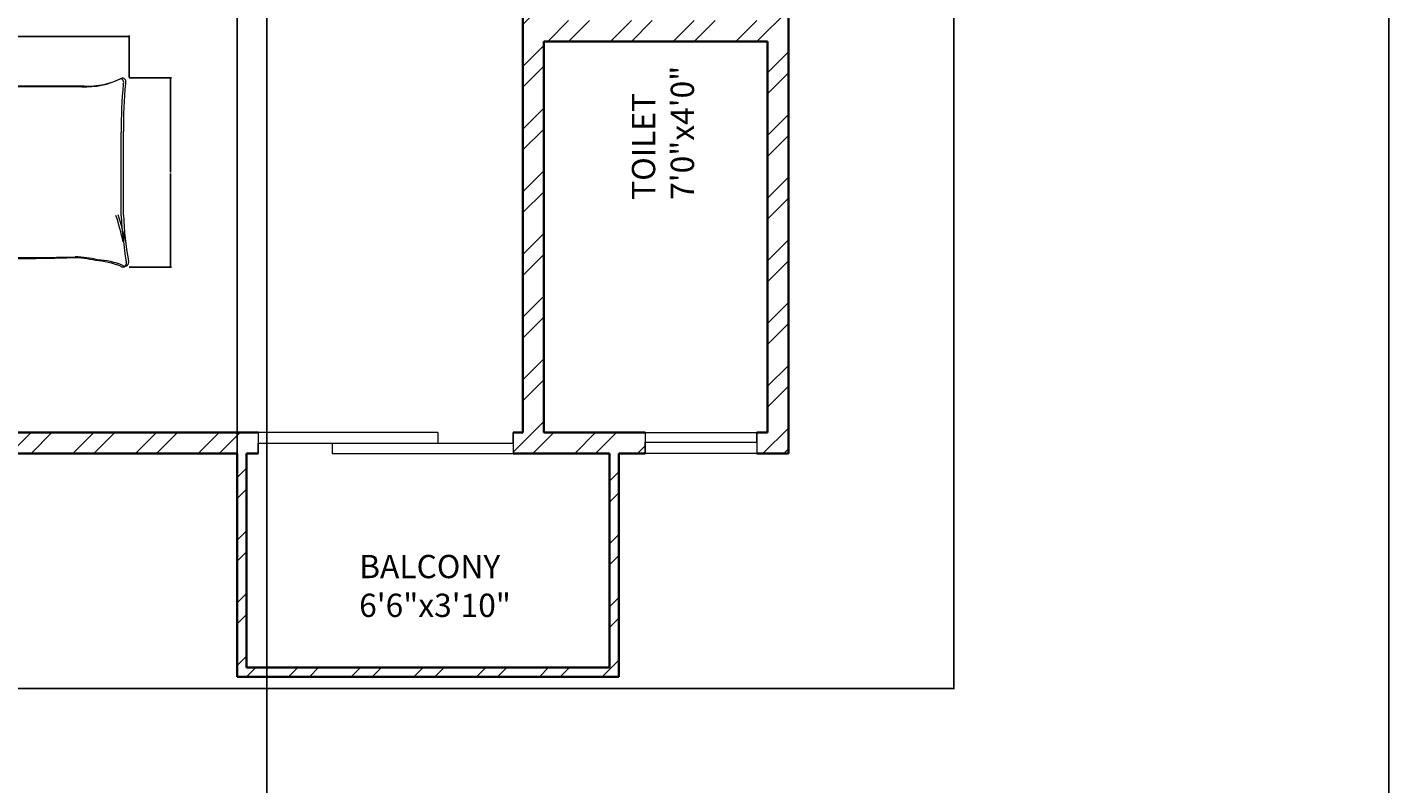
# Model space of a CAD drawing. Units: inches. Extents: x 2064 to 2782, y 1196 to 2299.
# Tile 9 of 11: x 2490 to 2782, y 1620 to 1783. Entities that reach past the tile are written whole.
import ezdxf

# ---------------------------------------------------------------- set-up
doc = ezdxf.new("R2010")
doc.units = ezdxf.units.IN
for name, color, linetype, lineweight in [('A-ANNO-DIMS', 2, 'Continuous', 18), ('A-ANNO-TTLB', 7, 'Continuous', 25), ('A-AREA-IDEN', 7, 'Continuous', 18), ('A-FURN', 8, 'Continuous', 13), ('A-GLAZ', 151, 'Continuous', 18), ('A-WALL', 7, 'Continuous', 35), ('A-WALL-PATT', 9, 'Continuous', 13)]:
    doc.layers.add(name, color=color, linetype=linetype, lineweight=lineweight)
doc.styles.get("Standard").update_dxf_attribs({"font": 'arial.ttf'})
doc.dimstyles.get("Standard").update_dxf_attribs({"dimtxt": 0.18, "dimasz": 0.18, "dimexe": 0.18, "dimexo": 0.0625, "dimgap": 0.09, "dimtad": 0, "dimtih": 1, "dimtoh": 1, "dimdec": 4, "dimzin": 0, "dimdsep": 46, "dimtxsty": 'Standard', "dimcen": 0.09, "dimadec": 0, "dimazin": 0, "dimtfac": 1, "dimtdec": 4, "dimtofl": 0, "dimtmove": 0, "dimatfit": 3, "dimfxl": 1, "dimtolj": 1, "dimtzin": 0, "dimarcsym": 0})

# ---------------------------------------------------------------- blocks, each defined once
blk = doc.blocks.new('BED-DOUBLE')
for p, q in [((2.53, 46.14), (2.53, 59.33)), ((2.53, 46.14), (2.53, 59.33)), ((2.53, 59.33), (37.35, 59.33)), ((2.7, 45.67), (2.7, 58.87)), ((2.7, 45.67), (2.7, 58.87)), ((37.35, 59.33), (37.35, 39.95)), ((37.35, 59.33), (37.35, 39.95)), ((37.52, 59.33), (37.52, 58.87)), ((37.52, 58.87), (37.52, 39.48)), ((37.52, 58.87), (37.52, 39.48)), ((2.53, 58.22), (37.35, 58.22)), ((2.53, 58.22), (37.35, 58.22)), ((2.7, 57.75), (37.52, 57.75)), ((2.7, 57.75), (37.52, 57.75)), ((2.84, 56.9), (5.96, 57.14)), ((2.84, 56.9), (5.96, 57.14)), ((2.84, 56.92), (3.26, 54.6)), ((2.84, 56.92), (3.26, 54.6)), ((3, 56.45), (3.43, 54.14)), ((3, 56.45), (3.43, 54.14)), ((3.01, 56.44), (6.13, 56.68)), ((3.01, 56.44), (6.13, 56.68)), ((5.96, 57.14), (6.04, 57.13)), ((5.96, 57.14), (6.04, 57.13)), ((6.04, 57.13), (8.82, 56.92)), ((6.04, 57.13), (8.82, 56.92)), ((6.13, 56.68), (6.2, 56.66)), ((6.13, 56.68), (6.2, 56.66)), ((6.2, 56.66), (8.99, 56.45)), ((6.2, 56.66), (8.99, 56.45)), ((8.82, 56.92), (12.82, 56.18)), ((8.82, 56.92), (12.82, 56.18)), ((8.99, 56.45), (12.99, 55.72)), ((8.99, 56.45), (12.99, 55.72)), ((10.82, 56.6), (12.3, 57.13)), ((10.82, 56.6), (12.3, 57.13)), ((10.99, 56.14), (12.46, 56.66)), ((10.99, 56.14), (12.46, 56.66)), ((12.3, 57.13), (14.4, 57.66)), ((12.3, 57.13), (14.4, 57.66)), ((12.46, 56.66), (14.57, 57.19)), ((12.46, 56.66), (14.57, 57.19)), ((14.4, 57.66), (14.64, 57.66)), ((14.4, 57.66), (14.64, 57.66)), ((14.57, 57.19), (14.8, 57.19)), ((14.57, 57.19), (14.8, 57.19)), ((14.64, 57.66), (17.88, 57.55)), ((14.64, 57.66), (17.88, 57.55)), ((14.8, 57.19), (18.04, 57.09)), ((14.8, 57.19), (18.04, 57.09)), ((17.88, 57.55), (18.93, 57.97)), ((17.88, 57.55), (18.93, 57.97)), ((18.04, 57.09), (19.1, 57.51)), ((18.04, 57.09), (19.1, 57.51)), ((18.93, 57.97), (19.35, 54.07)), ((18.93, 57.97), (19.35, 54.07)), ((19.1, 57.51), (19.52, 53.61)), ((19.1, 57.51), (19.52, 53.61)), ((20.38, 57.52), (20.2, 53.6)), ((20.38, 57.52), (20.21, 53.6)), ((20.55, 57.05), (20.37, 53.14)), ((20.55, 57.05), (20.37, 53.14)), ((21.46, 57.16), (20.38, 57.52)), ((21.46, 57.16), (20.38, 57.52)), ((21.63, 56.7), (20.55, 57.05)), ((21.63, 56.7), (20.55, 57.05)), ((24.69, 57.47), (21.46, 57.16)), ((24.69, 57.47), (21.46, 57.16)), ((24.85, 57.01), (21.63, 56.7)), ((24.85, 57.01), (21.63, 56.7)), ((24.92, 57.49), (24.69, 57.47)), ((24.92, 57.49), (24.69, 57.47)), ((25.09, 57.02), (24.85, 57.01)), ((25.09, 57.02), (24.85, 57.01)), ((27.05, 57.09), (24.92, 57.49)), ((27.05, 57.09), (24.92, 57.49)), ((27.22, 56.63), (25.09, 57.02)), ((27.22, 56.63), (25.09, 57.02)), ((30.54, 57.1), (26.59, 56.11)), ((30.54, 57.1), (26.59, 56.11)), ((30.7, 56.63), (26.75, 55.65)), ((30.7, 56.63), (26.75, 55.65)), ((28.56, 56.66), (27.05, 57.09)), ((28.56, 56.66), (27.05, 57.09)), ((28.73, 56.19), (27.22, 56.63)), ((28.73, 56.19), (27.22, 56.63)), ((33.3, 57.48), (30.54, 57.1)), ((33.3, 57.48), (30.54, 57.1)), ((33.47, 57.02), (30.7, 56.63)), ((33.47, 57.02), (30.7, 56.63)), ((36.51, 57.47), (32.57, 57.54)), ((32.57, 57.54), (33.3, 57.48)), ((36.51, 57.47), (32.57, 57.54)), ((32.57, 57.54), (33.3, 57.48)), ((36.68, 57.01), (32.74, 57.08)), ((32.74, 57.08), (33.47, 57.02)), ((36.67, 57.01), (32.74, 57.08)), ((32.74, 57.08), (33.47, 57.02)), ((36.51, 57.47), (36.23, 55.13)), ((36.51, 57.47), (36.23, 55.13)), ((36.68, 57.01), (36.4, 54.67)), ((36.67, 57.01), (36.4, 54.67)), ((3.26, 54.6), (2.94, 52.71)), ((3.26, 54.6), (2.94, 52.71)), ((2.94, 52.71), (3.36, 51.97)), ((2.94, 52.71), (3.36, 51.97)), ((3.43, 54.14), (3.11, 52.24)), ((3.43, 54.14), (3.11, 52.24)), ((3.26, 50.18), (3.68, 52.81)), ((3.26, 50.18), (3.68, 52.81)), ((3.68, 52.81), (4.42, 54.81)), ((3.68, 52.81), (4.42, 54.81)), ((3.85, 52.34), (4.58, 54.35)), ((3.85, 52.34), (4.58, 54.35)), ((19.35, 54.07), (19.77, 51.76)), ((19.35, 54.07), (19.77, 51.76)), ((19.52, 53.61), (19.94, 51.29)), ((19.52, 53.61), (19.94, 51.29)), ((20.21, 53.6), (19.93, 51.26)), ((20.2, 53.6), (19.93, 51.26)), ((20.37, 53.14), (20.1, 50.8)), ((20.37, 53.14), (20.1, 50.8)), ((35.92, 53.32), (35.06, 55.27)), ((35.92, 53.32), (35.06, 55.27)), ((36.09, 52.85), (35.23, 54.8)), ((36.09, 52.85), (35.23, 54.8)), ((36.51, 50.72), (35.92, 53.32)), ((36.51, 50.72), (35.92, 53.32)), ((36.68, 50.25), (36.09, 52.85)), ((36.67, 50.25), (36.09, 52.85)), ((36.23, 55.13), (36.67, 53.26)), ((36.23, 55.13), (36.67, 53.26)), ((36.67, 53.26), (36.29, 52.5)), ((36.67, 53.26), (36.29, 52.5)), ((36.4, 54.67), (36.83, 52.79)), ((36.4, 54.67), (36.83, 52.79)), ((36.83, 52.79), (36.46, 52.03)), ((36.83, 52.79), (36.46, 52.03)), ((3.11, 52.24), (3.53, 51.5)), ((3.11, 52.24), (3.53, 51.5)), ((3.47, 49.02), (3.26, 50.18)), ((3.47, 49.02), (3.26, 50.18)), ((3.43, 49.71), (3.85, 52.34)), ((3.43, 49.71), (3.85, 52.34)), ((3.64, 48.55), (3.43, 49.71)), ((3.64, 48.55), (3.43, 49.71)), ((19.77, 50.81), (19.35, 49.44)), ((19.77, 50.81), (19.35, 49.44)), ((19.94, 50.34), (19.52, 48.97)), ((19.94, 50.34), (19.52, 48.97)), ((19.77, 51.76), (19.77, 50.81)), ((19.77, 51.76), (19.77, 50.81)), ((19.93, 51.26), (19.99, 50.32)), ((19.93, 51.26), (19.99, 50.32)), ((19.94, 51.29), (19.94, 50.34)), ((19.94, 51.29), (19.94, 50.34)), ((19.99, 50.32), (20.49, 48.98)), ((19.99, 50.32), (20.49, 48.98)), ((20.1, 50.8), (20.15, 49.85)), ((20.1, 50.8), (20.15, 49.85)), ((20.15, 49.85), (20.66, 48.51)), ((20.15, 49.85), (20.66, 48.51)), ((36.37, 49.55), (36.51, 50.72)), ((36.37, 49.55), (36.51, 50.72)), ((36.54, 49.08), (36.68, 50.25)), ((36.54, 49.08), (36.67, 50.25)), ((3.05, 46.7), (3.47, 49.02)), ((3.05, 46.7), (3.47, 49.02)), ((6.76, 47.23), (3.05, 46.7)), ((6.76, 47.23), (3.05, 46.7)), ((3.21, 46.24), (3.64, 48.55)), ((3.21, 46.24), (3.64, 48.55)), ((4.65, 47.95), (7.59, 47.46)), ((4.65, 47.95), (7.59, 47.46)), ((4.82, 47.48), (7.75, 47)), ((4.82, 47.48), (7.75, 47)), ((7.59, 47.46), (6.76, 47.23)), ((7.59, 47.46), (6.76, 47.23)), ((7.75, 47), (6.93, 46.76)), ((7.75, 47), (6.93, 46.76)), ((7.59, 47.46), (12.69, 47.15)), ((7.59, 47.46), (12.69, 47.15)), ((7.75, 47), (12.86, 46.68)), ((7.75, 47), (12.86, 46.68)), ((12.69, 47.15), (14.12, 47.55)), ((12.69, 47.15), (14.12, 47.55)), ((12.86, 46.68), (14.29, 47.09)), ((12.86, 46.68), (14.29, 47.09)), ((14.12, 47.55), (17.86, 47.26)), ((14.12, 47.55), (17.86, 47.26)), ((14.29, 47.09), (18.03, 46.79)), ((14.29, 47.09), (18.03, 46.79)), ((17.56, 47.49), (15.27, 48.28)), ((17.56, 47.49), (15.27, 48.28)), ((17.73, 47.02), (15.44, 47.82)), ((17.73, 47.02), (15.44, 47.82)), ((19.35, 47.49), (17.56, 47.49)), ((19.35, 47.49), (17.56, 47.49)), ((19.52, 47.02), (17.73, 47.02)), ((19.52, 47.02), (17.73, 47.02)), ((19.35, 49.44), (19.35, 47.49)), ((19.35, 49.44), (19.35, 47.49)), ((19.52, 48.97), (19.52, 47.02)), ((19.52, 48.97), (19.52, 47.02)), ((20.49, 48.98), (20.62, 47.03)), ((20.49, 48.98), (20.62, 47.03)), ((20.62, 47.03), (22.4, 47.14)), ((20.62, 47.03), (22.4, 47.14)), ((20.66, 48.51), (20.78, 46.56)), ((20.66, 48.51), (20.78, 46.56)), ((22.4, 47.14), (24.64, 48.08)), ((22.4, 47.14), (24.64, 48.08)), ((22.57, 46.67), (24.81, 47.61)), ((22.57, 46.67), (24.81, 47.61)), ((23.72, 47.95), (26.66, 47.46)), ((23.72, 47.95), (26.66, 47.46)), ((23.89, 47.48), (26.83, 47)), ((23.89, 47.48), (26.83, 47)), ((26.66, 47.46), (31.77, 47.15)), ((26.66, 47.46), (31.77, 47.15)), ((26.83, 47), (31.94, 46.68)), ((26.83, 47), (31.94, 46.68)), ((31.77, 47.15), (33.2, 47.55)), ((31.77, 47.15), (33.2, 47.55)), ((31.94, 46.68), (33.36, 47.09)), ((31.94, 46.68), (33.36, 47.09)), ((33.2, 47.55), (36.94, 47.26)), ((33.2, 47.55), (36.94, 47.26)), ((33.36, 47.09), (37.1, 46.79)), ((33.36, 47.09), (37.1, 46.79)), ((36.94, 47.26), (36.37, 49.55)), ((36.94, 47.26), (36.37, 49.55)), ((37.1, 46.79), (36.54, 49.08)), ((37.1, 46.79), (36.54, 49.08)), ((6.93, 46.76), (3.21, 46.24)), ((6.93, 46.76), (3.21, 46.24)), ((20.78, 46.56), (22.57, 46.67)), ((20.78, 46.56), (22.57, 46.67)), ((22.05, 46.67), (25.1, 41.94)), ((22.05, 46.67), (25.1, 41.94)), ((22.21, 46.2), (25.26, 41.47)), ((22.21, 46.2), (25.26, 41.47)), ((29.61, 44.53), (23.54, 46.67)), ((29.61, 44.53), (23.54, 46.67)), ((29.78, 44.07), (23.7, 46.2)), ((29.78, 44.07), (23.7, 46.2)), ((33.67, 43.07), (29.61, 44.53)), ((33.67, 43.07), (29.61, 44.53)), ((33.84, 42.6), (29.78, 44.07)), ((33.84, 42.6), (29.78, 44.07)), ((25.1, 41.94), (26.34, 38.67)), ((25.1, 41.94), (26.34, 38.67)), ((25.26, 41.47), (26.51, 38.2)), ((25.26, 41.47), (26.51, 38.2)), ((35.82, 41.49), (33.67, 43.07)), ((35.82, 41.49), (33.67, 43.07)), ((35.98, 41.02), (33.84, 42.6)), ((35.98, 41.02), (33.84, 42.6)), ((38.52, 39.12), (35.82, 41.49)), ((38.52, 39.12), (35.82, 41.49)), ((38.68, 38.65), (35.98, 41.02)), ((38.68, 38.65), (35.98, 41.02)), ((26.34, 38.67), (26.56, 37.2)), ((26.34, 38.67), (26.56, 37.2)), ((26.51, 38.2), (26.73, 36.74)), ((26.51, 38.2), (26.73, 36.74)), ((28.37, 37.65), (29.84, 38.33)), ((28.37, 37.65), (29.84, 38.33)), ((29.84, 38.33), (32.32, 38.67)), ((29.84, 38.33), (32.32, 38.67)), ((30, 37.87), (32.49, 38.2)), ((30, 37.87), (32.49, 38.2)), ((32.32, 38.67), (35.14, 38.9)), ((32.32, 38.67), (35.14, 38.9)), ((32.49, 38.2), (35.31, 38.43)), ((32.49, 38.2), (35.31, 38.43)), ((35.14, 38.9), (37.4, 38.67)), ((35.14, 38.9), (37.4, 38.67)), ((35.31, 38.43), (37.56, 38.2)), ((35.31, 38.43), (37.56, 38.2)), ((37.4, 38.67), (38.52, 39.12)), ((37.4, 38.67), (38.52, 39.12)), ((37.56, 38.2), (38.68, 38.65)), ((37.56, 38.2), (38.68, 38.65)), ((38.57, 37.85), (38.52, 39.12, 2.82)), ((38.57, 37.85), (38.52, 39.12, 2.82)), ((38.74, 37.38), (38.68, 38.65, 2.82)), ((38.74, 37.38), (38.68, 38.65, 2.82)), ((26.56, 37.2), (28.37, 37.65)), ((26.56, 37.2), (28.37, 37.65)), ((26.73, 36.74), (28.54, 37.19)), ((26.73, 36.74), (28.54, 37.19)), ((28.54, 37.19), (30, 37.87)), ((28.54, 37.19), (30, 37.87)), ((10.97, 1.6), (28.91, 1.6)), ((10.97, 1.6), (28.91, 1.6)), ((11.14, 1.14), (29.07, 1.14)), ((11.14, 1.14), (29.07, 1.14))]:
    blk.add_line(p, q)
for centre, radius, start, end in [((15.56, -73.3), 120.19, 86.0865, 96.7821), ((15.56, -73.3), 120.19, 86.0865, 96.7821), ((62.04, 44.69), 60.69, 178.7218, 185.604), ((62.04, 44.69), 60.69, 178.7218, 185.604), ((62.21, 44.23), 60.69, 178.7218, 185.604), ((62.21, 44.23), 60.69, 178.7218, 185.604), ((15.73, -73.76), 120.19, 86.0865, 96.7821), ((15.73, -73.76), 120.19, 86.0865, 96.7821), ((12.94, -54.55), 94, 81.7845, 96.9006), ((12.94, -54.55), 94, 81.7845, 96.9006), ((13.1, -55.01), 94, 81.7845, 96.9006), ((13.1, -55.01), 94, 81.7845, 96.9006), ((-121.89, 36.62), 123.93, 358.4762, 1.0082), ((-121.89, 36.62), 123.93, 358.4762, 1.0082), ((-121.72, 36.16), 123.93, 358.4762, 1.0082), ((-121.72, 36.16), 123.93, 358.4762, 1.0082), ((31.87, 33.79), 4.53, 78.6608, 113.7384), ((31.87, 33.79), 4.53, 78.6608, 113.7384), ((37.39, 64.18), 26.36, 259.8763, 272.5657), ((37.39, 64.18), 26.36, 259.8763, 272.5657), ((26.69, 37.16), 0.134, 160.2464, 271.1377), ((26.69, 37.16), 0.134, 160.2464, 271.1377), ((22.7, 58.25), 21.6, 280.6617, 289.8806), ((22.7, 58.25), 21.6, 280.6617, 289.8806), ((26.86, 36.69), 0.134, 160.2464, 271.1377), ((26.86, 36.69), 0.134, 160.2464, 271.1377), ((22.86, 57.79), 21.6, 280.6617, 289.8806), ((22.86, 57.79), 21.6, 280.6617, 289.8806), ((32.04, 33.32), 4.53, 78.6608, 113.7384), ((32.04, 33.32), 4.53, 78.6608, 113.7384), ((37.56, 63.72), 26.36, 259.8763, 272.5657), ((37.56, 63.72), 26.36, 259.8763, 272.5657), ((132.79, 32.88), 94.35, 176.9791, 183.8365), ((132.79, 32.88), 94.35, 176.9791, 183.8365), ((132.95, 32.41), 94.35, 176.9791, 183.8365), ((132.95, 32.41), 94.35, 176.9791, 183.8365), ((353.21, 22.46), 351.38, 178.2277, 181.7185), ((353.21, 22.46), 351.38, 178.2277, 181.7185), ((353.38, 21.99), 351.38, 178.2277, 181.7185), ((353.38, 21.99), 351.38, 178.2277, 181.7185), ((-3284.8, 9.92), 3323.5, 0.00217, 0.28689), ((-3284.8, 9.92), 3323.5, 0.00217, 0.28689), ((-3284.64, 9.46), 3323.5, 0.00217, 0.28689), ((-3284.64, 9.46), 3323.5, 0.00217, 0.28689), ((-19.6, 12.33), 21.59, 346.0648, 358.9113), ((-19.6, 12.33), 21.59, 346.0648, 358.9113), ((-19.43, 11.87), 21.59, 346.0648, 358.9113), ((-19.43, 11.87), 21.59, 346.0648, 358.9113), ((55.48, 9.31), 16.8, 177.4714, 206.4681), ((55.48, 9.31), 16.8, 177.4714, 206.4681), ((55.65, 8.84), 16.8, 177.4714, 206.4681), ((55.65, 8.84), 16.8, 177.4714, 206.4681), ((-15.78, 8.14), 17.17, 337.9751, 356.652), ((-15.78, 8.14), 17.17, 337.9751, 356.652), ((-15.61, 7.67), 17.17, 337.9751, 356.652), ((-15.61, 7.67), 17.17, 337.9751, 356.652), ((0.79, 1.26), 0.793, 146.1736, 293.4781), ((0.79, 1.26), 0.793, 146.1736, 293.4781), ((0.96, 0.79), 0.793, 146.1736, 293.4781), ((0.96, 0.79), 0.793, 146.1736, 293.4781), ((15.61, -86.98), 88.71, 92.9958, 99.4091), ((15.61, -86.98), 88.71, 92.9958, 99.4091), ((15.78, -87.45), 88.71, 92.9958, 99.4091), ((15.78, -87.45), 88.71, 92.9958, 99.4091), ((-12.55, 76.61), 77.56, 283.3832, 287.7053), ((-12.55, 76.61), 77.56, 283.3832, 287.7053), ((-12.38, 76.14), 77.56, 283.3832, 287.7053), ((-12.38, 76.14), 77.56, 283.3832, 287.7053), ((29.98, -95.32), 96.92, 84.4998, 90.6351), ((29.98, -95.32), 96.92, 84.4998, 90.6351), ((30.15, -95.78), 96.92, 84.4998, 90.6351), ((30.15, -95.78), 96.92, 84.4998, 90.6351), ((39.64, 1.87), 0.803, 242.6588, 356.02), ((39.64, 1.87), 0.803, 242.6588, 356.02), ((39.81, 1.41), 0.803, 242.6588, 356.02), ((39.81, 1.41), 0.803, 242.6588, 356.02)]:
    blk.add_arc(centre, radius, start, end)
blk = doc.blocks.new('*D8')
at = {"layer": 'A-ANNO-DIMS', "color": 0, "lineweight": -2, "transparency": 16777216}
for p, q in [((2452.17, 1772.06), (2452.17, 1781.09)), ((2452.35, 1780.91), (2480.51, 1780.91)), ((2511.4, 1780.91), (2483.24, 1780.91)), ((2511.58, 1772.06), (2511.58, 1781.09))]:
    blk.add_line(p, q, dxfattribs=at)
at = {"layer": 'A-ANNO-DIMS', "color": 0, "transparency": 16777216}
for points in [[(2452.35, 1780.94), (2452.35, 1780.88), (2452.17, 1780.91)], [(2511.4, 1780.94), (2511.4, 1780.88), (2511.58, 1780.91)]]:
    blk.add_solid(points, dxfattribs=at)
at = {"layer": 'Defpoints', "color": 0, "transparency": 16777216}
for p in [(2452.17, 1780.91), (2452.17, 1771.99), (2511.58, 1771.99)]:
    blk.add_point(p, dxfattribs=at)
at = {"layer": 'A-ANNO-DIMS', "color": 0, "transparency": 16777216, "insert": (2481.87, 1780.91), "char_height": 0.18, "attachment_point": 5}
blk.add_mtext('\\A1;DOUBLE BED 59 TYP.', dxfattribs=at)
blk = doc.blocks.new('*D9')
at = {"layer": 'A-ANNO-DIMS', "color": 0, "lineweight": -2, "transparency": 16777216}
for p, q in [((2511.64, 1771.99), (2520.67, 1771.99)), ((2520.49, 1771.81), (2520.49, 1751.84)), ((2520.49, 1731.5), (2520.49, 1751.48)), ((2511.64, 1731.32), (2520.67, 1731.32))]:
    blk.add_line(p, q, dxfattribs=at)
at = {"layer": 'A-ANNO-DIMS', "color": 0, "transparency": 16777216}
for points in [[(2520.46, 1771.81), (2520.52, 1771.81), (2520.49, 1771.99)], [(2520.46, 1731.5), (2520.52, 1731.5), (2520.49, 1731.32)]]:
    blk.add_solid(points, dxfattribs=at)
at = {"layer": 'Defpoints', "color": 0, "transparency": 16777216}
for p in [(2511.58, 1771.99), (2520.49, 1771.99), (2511.58, 1731.32)]:
    blk.add_point(p, dxfattribs=at)
at = {"layer": 'A-ANNO-DIMS', "color": 0, "transparency": 16777216, "insert": (2520.49, 1751.66), "char_height": 0.18, "attachment_point": 5}
blk.add_mtext('\\A1;41 TYP.', dxfattribs=at)
blk = doc.blocks.new('*D23')
at = {"layer": 'A-ANNO-DIMS', "color": 0, "lineweight": -2, "transparency": 16777216}
for p, q in [((2653.23, 2234.29), (2688.85, 2234.29)), ((2688.67, 2234.11), (2688.67, 1937.72)), ((2688.67, 1640.97), (2688.67, 1937.36)), ((2452.23, 1640.79), (2688.85, 1640.79))]:
    blk.add_line(p, q, dxfattribs=at)
at = {"layer": 'A-ANNO-DIMS', "color": 0, "transparency": 16777216}
for points in [[(2688.64, 2234.11), (2688.7, 2234.11), (2688.67, 2234.29)], [(2688.64, 1640.97), (2688.7, 1640.97), (2688.67, 1640.79)]]:
    blk.add_solid(points, dxfattribs=at)
at = {"layer": 'Defpoints', "color": 0, "transparency": 16777216}
for p in [(2653.17, 2234.29), (2688.67, 2234.29), (2452.17, 1640.79)]:
    blk.add_point(p, dxfattribs=at)
at = {"layer": 'A-ANNO-DIMS', "color": 0, "transparency": 16777216, "insert": (2688.67, 1937.54), "char_height": 0.18, "attachment_point": 5}
blk.add_mtext('\\A1;593.5', dxfattribs=at)
blk = doc.blocks.new('*D27')
at = {"layer": 'A-ANNO-DIMS', "color": 0, "lineweight": -2, "transparency": 16777216}
for p, q in [((2452.17, 1640.85), (2452.17, 2269.97)), ((2452.35, 2269.79), (2493.09, 2269.79)), ((2534.61, 2269.79), (2493.87, 2269.79)), ((2534.79, 1643.35), (2534.79, 2269.97))]:
    blk.add_line(p, q, dxfattribs=at)
at = {"layer": 'A-ANNO-DIMS', "color": 0, "transparency": 16777216}
for points in [[(2452.35, 2269.82), (2452.35, 2269.76), (2452.17, 2269.79)], [(2534.61, 2269.82), (2534.61, 2269.76), (2534.79, 2269.79)]]:
    blk.add_solid(points, dxfattribs=at)
at = {"layer": 'Defpoints', "color": 0, "transparency": 16777216}
for p in [(2534.79, 2269.79), (2534.79, 1643.29), (2452.17, 1640.79)]:
    blk.add_point(p, dxfattribs=at)
at = {"layer": 'A-ANNO-DIMS', "color": 0, "transparency": 16777216, "insert": (2493.48, 2269.79), "char_height": 0.18, "attachment_point": 5}
blk.add_mtext('\\A1;82.62', dxfattribs=at)
blk = doc.blocks.new('*D36')
at = {"layer": 'A-ANNO-DIMS', "color": 0, "lineweight": -2, "transparency": 16777216}
for p, q in [((2390.62, 2058.73), (2390.62, 1539.01)), ((2541.17, 2058.73), (2541.17, 1539.01)), ((2390.8, 1539.19), (2465.44, 1539.19)), ((2540.99, 1539.19), (2466.35, 1539.19))]:
    blk.add_line(p, q, dxfattribs=at)
at = {"layer": 'A-ANNO-DIMS', "color": 0, "transparency": 16777216}
for points in [[(2390.8, 1539.22), (2390.8, 1539.16), (2390.62, 1539.19)], [(2540.99, 1539.22), (2540.99, 1539.16), (2541.17, 1539.19)]]:
    blk.add_solid(points, dxfattribs=at)
at = {"layer": 'Defpoints', "color": 0, "transparency": 16777216}
for p in [(2390.62, 2058.79), (2541.17, 2058.79), (2541.17, 1539.19)]:
    blk.add_point(p, dxfattribs=at)
at = {"layer": 'A-ANNO-DIMS', "color": 0, "transparency": 16777216, "insert": (2465.9, 1539.19), "char_height": 0.18, "attachment_point": 5}
blk.add_mtext('\\A1;150.55', dxfattribs=at)

msp = doc.modelspace()

# ---------------------------------------------------------------- hatches: boundary and pattern name
at = {"layer": 'A-WALL-PATT'}
h = msp.add_hatch(dxfattribs=at)
h.set_pattern_fill('ANSI32', color=256)
h.paths.add_polyline_path([(2489.7688, 2189.2917), (2574.5454, 2189.2917), (2574.5454, 2191.5417), (2574.5454, 2193.7917), (2570.6691, 2193.7917), (2570.6691, 2197.3052), (2568.4191, 2197.3052), (2566.1691, 2197.3052), (2566.1691, 2193.7917), (2494.1691, 2193.7917), (2494.1691, 2229.7917), (2523.2441, 2229.7917), (2523.2441, 2234.2917), (2471.2886, 2234.2917), (2471.2886, 2229.7917), (2489.6691, 2229.7917), (2489.6691, 2193.7917), (2417.6691, 2193.7917), (2417.6691, 2197.0632), (2415.4191, 2197.0632), (2413.1691, 2197.0632), (2413.1691, 2193.7917), (2406.8865, 2193.7917), (2406.8865, 2189.2917), (2485.2688, 2189.2917), (2485.2688, 2063.2917), (2369.1629, 2063.2917), (2369.1629, 2058.7917), (2386.1222, 2058.7917), (2386.1222, 1856.2917), (2382.1576, 1856.2917), (2382.1576, 1851.7917), (2394.9764, 1851.7917), (2394.9764, 1854.0417), (2394.9764, 1856.2917), (2390.6222, 1856.2917), (2390.6222, 2058.7917), (2485.2688, 2058.7917), (2493.762, 2058.7917), (2493.762, 2061.0417), (2493.762, 2063.2917), (2489.7688, 2063.2917)])
h.paths.add_polyline_path([(2447.2886, 2234.2917), (2413.1691, 2234.2917), (2413.1691, 2217.3799), (2417.6691, 2217.3799), (2417.6691, 2229.7917), (2447.2886, 2229.7917)], flags=17)
h.paths.add_polyline_path([(2570.6691, 2234.2917), (2547.2441, 2234.2917), (2547.2441, 2229.7917), (2566.1691, 2229.7917), (2566.1691, 2216.5615), (2570.6691, 2216.5615)], flags=17)
h.paths.add_polyline_path([(2653.1691, 2189.2917), (2653.1691, 2193.7917), (2640.8843, 2193.7917), (2640.8843, 2189.2917), (2648.6691, 2189.2917), (2648.6691, 2162.7138), (2653.1691, 2162.7138)])
h.paths.add_polyline_path([(2653.1691, 2102.7138), (2648.6691, 2102.7138), (2648.6691, 2063.2917), (2526.7281, 2063.2917), (2526.7281, 2058.7917), (2541.1691, 2058.7917), (2541.1691, 1993.2917), (2545.6691, 1993.2917), (2545.6691, 1997.7917), (2545.6691, 2058.7917), (2648.6691, 2058.7917), (2648.6691, 2050.1099), (2653.1691, 2050.1099)])
h.paths.add_polyline_path([(2600.6691, 1856.2917), (2493.4607, 1856.2917), (2493.4607, 1851.7917), (2596.1691, 1851.7917), (2596.1691, 1695.7917), (2594.0816, 1695.7917), (2594.0816, 1691.2917), (2614.7905, 1691.2917), (2614.7905, 1645.2917), (2536.7905, 1645.2917), (2536.7905, 1691.2917), (2539.332, 1691.2917), (2539.332, 1693.5417), (2539.332, 1695.7917), (2452.1691, 1695.7917), (2452.1691, 1851.7917), (2456.0775, 1851.7917), (2456.0775, 1856.2917), (2427.1536, 1856.2917), (2427.1536, 1851.7917), (2447.6691, 1851.7917), (2447.6691, 1695.7917), (2447.6691, 1645.2917), (2405.1469, 1645.2917), (2405.1469, 1640.7917), (2452.1691, 1640.7917), (2452.1691, 1645.2917), (2452.1691, 1691.2917), (2534.7905, 1691.2917), (2534.7905, 1645.2917), (2534.7905, 1643.2917), (2614.7905, 1643.2917), (2616.7905, 1643.2917), (2616.7905, 1691.2917), (2622.4029, 1691.2917), (2622.4029, 1693.7143), (2622.4029, 1695.7917), (2600.6691, 1695.7917), (2600.6691, 1779.7917), (2648.6691, 1779.7917), (2648.6691, 1695.7917), (2646.4029, 1695.7917), (2646.4029, 1691.2917), (2653.1691, 1691.2917), (2653.1691, 1906.3508), (2648.6691, 1906.3508), (2648.6691, 1856.2917), (2648.6691, 1784.2917), (2600.6691, 1784.2917)])
h.paths.add_polyline_path([(2322.9532, 1819.5181), (2320.7032, 1819.5181), (2318.4532, 1819.5181), (2318.4532, 1695.7917), (2242.7664, 1695.7917), (2242.7664, 1691.2917), (2318.4532, 1691.2917), (2318.4532, 1640.7917), (2322.9532, 1640.7917), (2345.1469, 1640.7917), (2345.1469, 1643.0417), (2345.1469, 1645.2917), (2322.9532, 1645.2917), (2322.9532, 1691.2917), (2322.9532, 1695.7917)])
h.paths.add_polyline_path([(2166.1825, 1691.2917), (2164.1825, 1691.2917), (2164.1825, 1643.2917), (2166.1825, 1643.2917), (2246.1825, 1643.2917), (2246.1825, 1645.2917), (2246.1825, 1691.2917), (2244.1825, 1691.2917), (2244.1825, 1645.2917), (2166.1825, 1645.2917)])
h.paths.add_polyline_path([(2309.404, 1932.7917), (2204.1691, 1932.7917), (2204.1691, 1960.0962), (2199.6691, 1960.0962), (2199.6691, 1932.7917), (2132.6691, 1932.7917), (2132.6691, 1951.0737), (2128.1691, 1951.0737), (2128.1691, 1910.0412), (2132.6691, 1910.0412), (2132.6691, 1928.2917), (2304.904, 1928.2917), (2304.904, 1856.2917), (2304.904, 1851.7917), (2318.4532, 1851.7917), (2318.4532, 1848.8308), (2322.9532, 1848.8308), (2322.9532, 1851.7917), (2347.7631, 1851.7917), (2347.7631, 1856.2917), (2309.404, 1856.2917)])
h.paths.add_polyline_path([(2132.6691, 2044.9092), (2130.4191, 2044.9092), (2128.1691, 2044.9092), (2128.1691, 1987.0737), (2132.6691, 1987.0737), (2132.6691, 2004.7917), (2199.6691, 2004.7917), (2204.1691, 2004.7917), (2204.1691, 2009.2917), (2132.6691, 2009.2917)])
h.paths.add_polyline_path([(2186.6691, 2195.9329), (2184.4191, 2195.9329), (2184.4191, 2195.8929), (2182.1691, 2195.9329), (2182.1691, 2193.7917), (2128.1691, 2193.7917), (2128.1691, 2181.4967), (2132.6691, 2181.4967), (2132.6691, 2182.7769), (2132.6691, 2189.2917), (2182.1691, 2189.2917), (2182.1691, 2135.2917), (2179.804, 2135.2917), (2179.804, 2130.7917), (2190.215, 2130.7917), (2190.215, 2133.0417), (2190.215, 2135.2917), (2186.6691, 2135.2917)])
h.paths.add_polyline_path([(2340.0628, 2189.2917), (2340.0628, 2191.5417), (2340.0628, 2193.7917), (2335.1691, 2193.7917), (2335.1691, 2234.2917), (2280.6746, 2234.2917), (2280.6746, 2229.7917), (2330.6691, 2229.7917), (2330.6691, 2193.7917), (2330.6691, 2135.2917), (2218.6309, 2135.2917), (2218.6309, 2130.7917), (2330.7688, 2130.7917), (2330.7688, 2008.4023), (2335.2688, 2008.4023), (2335.2688, 2058.7917), (2338.9208, 2058.7917), (2338.9208, 2061.0417), (2338.9208, 2063.2917), (2335.2688, 2063.2917), (2335.2688, 2189.2917)])
h.paths.add_polyline_path([(2220.6746, 2234.2917), (2182.1691, 2234.2917), (2182.1691, 2227.4187), (2186.6691, 2227.4187), (2186.6691, 2229.7917), (2220.6746, 2229.7917), (2220.6746, 2232.0417)])
h.paths.add_polyline_path([(2158.8146, 2135.2917), (2132.6691, 2135.2917), (2132.6691, 2157.4967), (2128.1691, 2157.4967), (2128.1691, 2104.9092), (2132.6691, 2104.9092), (2132.6691, 2130.7917), (2158.8146, 2130.7917), (2158.8146, 2133.0417)])
h.paths.add_polyline_path([(2396.0464, 2062.2045), (2434.8868, 2062.2045), (2434.8868, 2080.8619), (2396.0464, 2080.8619)], flags=24)
h.paths.add_polyline_path([(2196.1396, 1653.3449), (2232.023, 1653.3449), (2232.023, 1672.0022), (2196.1396, 1672.0022)], flags=25)

# ---------------------------------------------------------------- linework, layer by layer
at = {"layer": 'A-ANNO-TTLB'}
msp.add_lwpolyline([(2063.9994, 2298.574), (2782.0941, 2298.574), (2782.0941, 1490.6238), (2063.9994, 1490.6238)], close=True, dxfattribs=at)
at = {"layer": 'A-GLAZ'}
for p, q in [((2539.332, 1695.7917), (2539.332, 1691.2917)), ((2577.8798, 1695.7917), (2539.332, 1695.7917)), ((2577.8798, 1695.7917), (2577.8798, 1693.5417)), ((2594.0816, 1693.5417), (2594.0816, 1695.7917)), ((2594.0816, 1695.7917), (2594.0816, 1691.2917)), ((2622.4029, 1695.7917), (2622.4029, 1691.2917)), ((2622.4029, 1695.7917), (2646.4029, 1695.7917)), ((2646.4029, 1693.7143), (2646.4029, 1695.7917)), ((2646.4029, 1695.7917), (2646.4029, 1691.2917)), ((2539.332, 1691.2917), (2539.332, 1693.5417)), ((2539.332, 1693.5417), (2594.0816, 1693.5417)), ((2555.2119, 1693.5417), (2555.2119, 1691.2917)), ((2622.4029, 1691.2917), (2622.4029, 1693.7143)), ((2622.4029, 1693.7143), (2646.4029, 1693.7143)), ((2555.2119, 1691.2917), (2594.0816, 1691.2917)), ((2646.4029, 1691.2917), (2622.4029, 1691.2917))]:
    msp.add_line(p, q, dxfattribs=at)
at = {"layer": 'A-WALL'}
for p, q in [((2653.1691, 1906.3508), (2653.1691, 1691.2917)), ((2596.1691, 1695.7917), (2596.1691, 1851.7917)), ((2600.6691, 1695.7917), (2600.6691, 1779.7917)), ((2600.6691, 1779.7917), (2648.6691, 1779.7917)), ((2648.6691, 1695.7917), (2648.6691, 1779.7917)), ((2452.1691, 1695.7917), (2539.332, 1695.7917)), ((2594.0816, 1695.7917), (2596.1691, 1695.7917)), ((2600.6691, 1695.7917), (2622.4029, 1695.7917)), ((2646.4029, 1695.7917), (2648.6691, 1695.7917)), ((2452.1691, 1691.2917), (2534.7905, 1691.2917)), ((2534.7905, 1691.2917), (2534.7905, 1645.2917)), ((2536.7905, 1645.2917), (2536.7905, 1691.2917)), ((2536.7905, 1691.2917), (2539.332, 1691.2917)), ((2594.0816, 1691.2917), (2614.7905, 1691.2917)), ((2614.7905, 1691.2917), (2614.7905, 1645.2917)), ((2616.7905, 1643.2917), (2616.7905, 1691.2917)), ((2616.7905, 1691.2917), (2622.4029, 1691.2917)), ((2646.4029, 1691.2917), (2653.1691, 1691.2917)), ((2534.7905, 1645.2917), (2534.7905, 1643.2917)), ((2534.7905, 1643.2917), (2614.7905, 1643.2917)), ((2614.7905, 1645.2917), (2536.7905, 1645.2917)), ((2614.7905, 1643.2917), (2616.7905, 1643.2917))]:
    msp.add_line(p, q, dxfattribs=at)

# ---------------------------------------------------------------- block references
at = {"layer": 'A-FURN', "rotation": 89.99999983318565}
msp.add_blockref('BED-DOUBLE', (2511.5038, 1731.3857), dxfattribs=at)

# ---------------------------------------------------------------- texts
at = {"layer": 'A-AREA-IDEN', "insert": (2619.5662, 1745.7996), "char_height": 5, "attachment_point": 1, "rotation": 90}
msp.add_mtext_dynamic_manual_height_columns('TOILET\\P7\'0"x4\'0"', width=293.906283, gutter_width=12.5, heights=[0], dxfattribs=at)
at = {"layer": 'A-AREA-IDEN', "insert": (2560.9951, 1669.5176), "char_height": 5, "attachment_point": 1}
msp.add_mtext_dynamic_manual_height_columns('BALCONY\\P6\'6"x3\'10"', width=113.979526, gutter_width=12.5, heights=[0], dxfattribs=at)

# ---------------------------------------------------------------- dimensions: what is measured, and where the dimension line sits
at = {"layer": 'A-ANNO-DIMS'}
for base, p1, p2, picture, middle in [((2534.7905, 2269.7917), (2452.1691, 1640.7917), (2534.7905, 1643.2917), '*D27', (2493.4798, 2269.7917)), ((2541.1691, 1539.1896), (2390.6222, 2058.7917), (2541.1691, 2058.7917), '*D36', (2465.8957, 1539.1896))]:
    dim = msp.add_linear_dim(base=base, p1=p1, p2=p2, dimstyle='Standard', override={"dimdec": 2, "dimlfac": 1, "dimrnd": 0, "dimzin": 0, "dimdsep": 46, "dimlunit": 2}, dxfattribs=at)
    dim.commit()
    dim.dimension.update_dxf_attribs({"geometry": picture, "text_midpoint": middle})
dim = msp.add_linear_dim(base=(2688.6691, 2234.2917), p1=(2452.1691, 1640.7917), p2=(2653.1691, 2234.2917), angle=90, dimstyle='Standard', override={"dimdec": 1, "dimlfac": 1, "dimrnd": 0, "dimzin": 0, "dimdsep": 46, "dimlunit": 2}, dxfattribs=at)
dim.commit()
dim.dimension.update_dxf_attribs({"geometry": '*D23', "text_midpoint": (2688.6691, 1937.5417)})
for base, p1, p2, angle, text, picture, middle in [((2452.1691, 1780.905), (2511.5806, 1771.9933), (2452.1691, 1771.9933), 180, 'DOUBLE BED <> TYP.', '*D8', (2481.8748, 1780.905)), ((2520.4923, 1771.9933), (2511.5806, 1731.3228), (2511.5806, 1771.9933), 90, '<> TYP.', '*D9', (2520.4923, 1751.6581))]:
    dim = msp.add_linear_dim(base=base, p1=p1, p2=p2, angle=angle, text=text, dimstyle='Standard', override={"dimdec": 0, "dimlfac": 1, "dimrnd": 0, "dimzin": 0, "dimdsep": 46, "dimlunit": 2}, dxfattribs=at)
    dim.commit()
    dim.dimension.update_dxf_attribs({"geometry": picture, "text_midpoint": middle})

doc.saveas('drawing.dxf')
